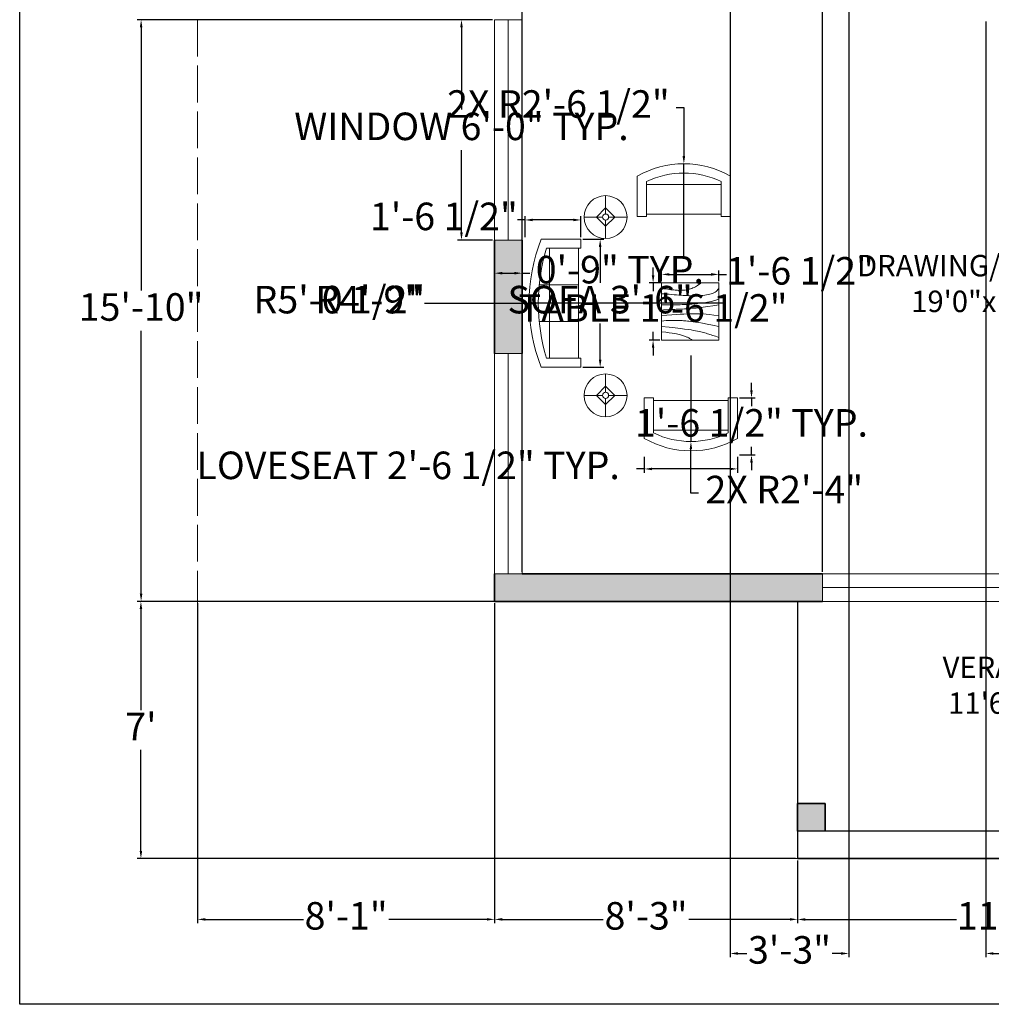
# Model space of a CAD drawing. Units: inches. Extents: x 1942 to 2601, y 2026 to 2623.
# Tile 1 of 5: x 1942 to 2259, y 2026 to 2348. Entities that reach past the tile are written whole.
import ezdxf

# ---------------------------------------------------------------- set-up
doc = ezdxf.new("R2010")
doc.units = ezdxf.units.IN
doc.linetypes.add('ACAD_ISO02W100', pattern=[15, 12, -3])
for name, color, linetype, lineweight in [('A-ANNO-DIMS', 2, 'Continuous', 18), ('A-ANNO-TTLB', 7, 'Continuous', 25), ('A-AREA-IDEN', 7, 'Continuous', 25), ('A-COLS', 7, 'Continuous', 35), ('A-FLOR', 7, 'Continuous', 25), ('A-FLOR-OTLN', 8, 'ACAD_ISO02W100', 13), ('A-FURN', 8, 'Continuous', 18), ('A-GLAZ', 2, 'Continuous', 18), ('A-WALL', 7, 'Continuous', 35), ('A-WALL-PATT', 7, 'Continuous', 13)]:
    doc.layers.add(name, color=color, linetype=linetype, lineweight=lineweight)
doc.styles.get("Standard").update_dxf_attribs({"font": 'arial.ttf'})
doc.dimstyles.new('ISO-25', dxfattribs={"dimtxt": 9, "dimasz": 2.5, "dimexe": 1.25, "dimexo": 0.625, "dimgap": 2, "dimtad": 0, "dimtih": 1, "dimtoh": 1, "dimdec": 1, "dimlunit": 4, "dimtxsty": 'Standard', "dimcen": 2.5, "dimadec": 0, "dimazin": 0, "dimtfac": 0.5, "dimtdec": 1, "dimtmove": 0, "dimatfit": 3, "dimfxl": 1, "dimarcsym": 0})

# ---------------------------------------------------------------- blocks, each defined once
blk = doc.blocks.new('Sofa - Roundback 7 ft.')
for p, q in [((-36.000027, -34), (-36.000027, -11.4696)), ((-12.00002, -32.4421), (-12.00003, -6.5971)), ((11.99997, -32.4421), (11.99998, -6.5971)), ((35.99998, -34), (35.99998, -11.4696)), ((-35.999844, -13.3819), (35.9998, -13.3819)), ((-36.000027, -32.4421), (35.99998, -32.4421))]:
    blk.add_line(p, q)
for points in [[(-36.000027, -34), (-42.000027, -34), (-42.000027, -8)], [(41.99998, -8), (41.99998, -34), (35.99998, -34)]]:
    blk.add_lwpolyline(points)
for centre, radius, start, end in [((0, -114.25), 114.25, 68.43141, 111.5686), ((-0.00001, -127.1968), 121.1968, 72.72033, 107.2797)]:
    blk.add_arc(centre, radius, start, end)
blk = doc.blocks.new('Sofa - Roundback Loveseat 5 ft.')
for p, q in [((0, -32.44198), (0, -5.99998)), ((-24, -33.99998), (-24, -11.46958)), ((24.00004, -33.99998), (24.00004, -11.46958)), ((-23.9998, -13.38178), (23.99986, -13.38178)), ((-24, -32.44198), (24.00004, -32.44198))]:
    blk.add_line(p, q)
for points in [[(-24, -33.99998), (-30, -33.99998), (-30, -7.99998)], [(30.00004, -7.99998), (30.00004, -33.99998), (24.00004, -33.99998)]]:
    blk.add_lwpolyline(points)
for centre, radius, start, end in [((0, -60.24998), 60.24998, 60.13715, 119.8628), ((0, -61.38438), 55.38444, 64.32083, 115.6792)]:
    blk.add_arc(centre, radius, start, end)
blk = doc.blocks.new('Table - Square Woodgrain 42 x 42 in.')
blk.add_line((0, -42), (42, -42))
for points in [[(0, -4), (1.704, -4.2172), (3.2358, -4.4188), (4.615, -4.604), (5.8615, -4.7721), (6.9951, -4.9224), (8.0357, -5.0541), (9.0031, -5.1667), (9.9171, -5.2594), (10.7951, -5.3316), (11.6445, -5.3836), (12.4702, -5.4157), (13.277, -5.4283), (14.0698, -5.4217), (14.8535, -5.3964), (15.6331, -5.3526), (16.4133, -5.2908), (17.1986, -5.2103), (17.9913, -5.1062), (18.793, -4.9727), (19.6056, -4.8038), (20.4307, -4.5937), (21.2701, -4.3365), (22.1256, -4.0262), (22.9989, -3.6571), (23.888, -3.2272), (24.7756, -2.7516), (25.6408, -2.2491), (26.4624, -1.7387), (27.2195, -1.2395), (27.891, -0.7703), (28.456, -0.3501), (28.8934, 0.002)], [(0, -42), (0, 0), (42, 0), (42, -42)], [(0, -8), (1.8203, -8.1001), (3.6741, -8.2149), (5.5411, -8.3408), (7.4011, -8.4741), (9.2339, -8.6112), (11.0193, -8.7484), (12.7371, -8.8821), (14.3671, -9.0086), (15.8954, -9.1246), (17.3337, -9.2278), (18.6997, -9.3159), (20.0116, -9.387), (21.2871, -9.4389), (22.5442, -9.4696), (23.8008, -9.477), (25.0749, -9.459), (26.3791, -9.4137), (27.7049, -9.3403), (29.0383, -9.2382), (30.3655, -9.1068), (31.6728, -8.9455), (32.9461, -8.7535), (34.1717, -8.5304), (35.3358, -8.2756), (36.4268, -7.9863), (37.443, -7.6521), (38.3849, -7.2603), (39.253, -6.7986), (40.048, -6.2542), (40.7705, -5.6147), (41.421, -4.8674), (42, -4)], [(42, -12), (39.1784, -12.8621), (36.4519, -13.5654), (33.8246, -14.1294), (31.3004, -14.5731), (28.8832, -14.9161), (26.577, -15.1775), (24.3858, -15.3768), (22.3136, -15.5332), (20.3622, -15.6632), (18.5254, -15.7718), (16.7947, -15.8612), (15.1618, -15.9338), (13.6183, -15.9916), (12.1558, -16.0369), (10.7659, -16.0718), (9.4403, -16.0987), (8.1703, -16.1191), (6.9461, -16.1325), (5.7577, -16.1377), (4.595, -16.1335), (3.4479, -16.1188), (2.3064, -16.0924), (1.1604, -16.0532), (0, -16)], [(42, -16), (37.6529, -16.7365), (33.8802, -17.329), (30.6179, -17.7961), (27.8015, -18.1561), (25.3668, -18.4275), (23.2497, -18.6288), (21.3859, -18.7785), (19.7111, -18.8949), (18.1693, -18.9939), (16.7375, -19.0795), (15.401, -19.1534), (14.1449, -19.217), (12.9544, -19.2717), (11.8148, -19.3191), (10.7113, -19.3606), (9.6291, -19.3976), (8.5534, -19.4323), (7.47, -19.4689), (6.3643, -19.5122), (5.222, -19.5672), (4.0288, -19.6386), (2.7703, -19.7313), (1.4321, -19.8501), (0, -20)], [(0, -24), (3.9243, -23.6805), (7.4766, -23.4138), (10.6891, -23.1954), (13.5943, -23.0205), (16.2247, -22.8847), (18.6125, -22.7832), (20.7903, -22.7116), (22.7903, -22.6651), (24.6563, -22.642), (26.4764, -22.6507), (28.35, -22.7024), (30.3766, -22.8084), (32.6555, -22.98), (35.2861, -23.2283), (38.3678, -23.5645), (42, -24)], [(42, -32), (37.392, -31.017), (33.4585, -30.2231), (30.1291, -29.5949), (27.3334, -29.109), (25.0009, -28.742), (23.0612, -28.4707), (21.4439, -28.2716), (20.0786, -28.1215), (18.8998, -28.0002), (17.8609, -27.9014), (16.9206, -27.8219), (16.0371, -27.7588), (15.1691, -27.709), (14.2748, -27.6693), (13.3128, -27.6368), (12.2415, -27.6083), (11.0295, -27.5824), (9.6867, -27.5643), (8.233, -27.5608), (6.6884, -27.5787), (5.0728, -27.6248), (3.4062, -27.7058), (1.7086, -27.8286), (0, -28)], [(0, -32), (5.4026, -32.5358), (9.9494, -33.019), (13.7424, -33.4553), (16.8834, -33.8505), (19.4743, -34.2106), (21.6171, -34.5413), (23.4136, -34.8486), (24.9657, -35.1382), (26.3614, -35.4156), (27.6332, -35.6841), (28.7995, -35.9467), (29.8788, -36.2064), (30.8897, -36.4661), (31.8507, -36.7288), (32.7802, -36.9973), (33.6968, -37.2747), (34.6175, -37.5635), (35.5531, -37.8651), (36.5128, -38.1805), (37.506, -38.5108), (38.5421, -38.8568), (39.6302, -39.2197), (40.7797, -39.6004), (42, -40)], [(0, -36), (3.0098, -36.2857), (5.5354, -36.5643), (7.6368, -36.8359), (9.374, -37.1009), (10.807, -37.3597), (11.9957, -37.6126), (13.0002, -37.8599), (13.8804, -38.102), (14.6874, -38.3393), (15.4365, -38.5729), (16.1338, -38.8041), (16.7858, -39.0341), (17.3987, -39.264), (17.9787, -39.4952), (18.5322, -39.7288), (19.0655, -39.9662), (19.5832, -40.2081), (20.0842, -40.4544), (20.5657, -40.7046), (21.0249, -40.9581), (21.459, -41.2144), (21.8653, -41.4731), (22.2409, -41.7335), (22.5831, -41.9951)]]:
    blk.add_lwpolyline(points)
blk = doc.blocks.new('Lamp - Table')
for p, q in [((0, 7), (0, 1)), ((-1, 0), (-7, 0)), ((0, 3), (-3, 0)), ((-3, 0), (0, -3)), ((3, 0), (0, 3)), ((0, -3), (3, 0)), ((1, 0), (7, 0)), ((0, -1), (0, -7))]:
    blk.add_line(p, q)
for radius in [7, 1]:
    blk.add_circle((0, 0), radius)
blk = doc.blocks.new('*D17')
at = {"layer": 'A-ANNO-DIMS', "color": 0, "lineweight": -2, "transparency": 16777216}
for p, q in [((2096.19, 2347.91), (1980.09, 2347.91)), ((1981.34, 2345.41), (1981.34, 2259.51)), ((1981.34, 2160.41), (1981.34, 2246.32)), ((2096.19, 2157.91), (1980.09, 2157.91))]:
    blk.add_line(p, q, dxfattribs=at)
at = {"layer": 'A-ANNO-DIMS', "color": 0, "transparency": 16777216}
for points in [[(1980.92, 2345.41), (1981.75, 2345.41), (1981.34, 2347.91)], [(1980.92, 2160.41), (1981.75, 2160.41), (1981.34, 2157.91)]]:
    blk.add_solid(points, dxfattribs=at)
at = {"layer": 'Defpoints', "color": 0, "transparency": 16777216}
for p in [(2096.82, 2347.91), (1981.34, 2157.91), (2096.82, 2157.91)]:
    blk.add_point(p, dxfattribs=at)
at = {"layer": 'A-ANNO-DIMS', "color": 0, "transparency": 16777216, "insert": (1981.34, 2252.91), "char_height": 9, "attachment_point": 5}
blk.add_mtext('15\'-10"', dxfattribs=at)
blk = doc.blocks.new('*D18')
at = {"layer": 'A-ANNO-DIMS', "color": 0, "lineweight": -2, "transparency": 16777216}
for p, q in [((2195.19, 2157.91), (1980.03, 2157.91)), ((1981.28, 2155.41), (1981.28, 2122.41)), ((1981.28, 2076.41), (1981.28, 2109.41)), ((2195.19, 2073.91), (1980.03, 2073.91))]:
    blk.add_line(p, q, dxfattribs=at)
at = {"layer": 'A-ANNO-DIMS', "color": 0, "transparency": 16777216}
for points in [[(1980.87, 2155.41), (1981.7, 2155.41), (1981.28, 2157.91)], [(1980.87, 2076.41), (1981.7, 2076.41), (1981.28, 2073.91)]]:
    blk.add_solid(points, dxfattribs=at)
at = {"layer": 'Defpoints', "color": 0, "transparency": 16777216}
for p in [(2195.82, 2157.91), (1981.28, 2073.91), (2195.82, 2073.91)]:
    blk.add_point(p, dxfattribs=at)
at = {"layer": 'A-ANNO-DIMS', "color": 0, "transparency": 16777216, "insert": (1981.28, 2115.91), "char_height": 9, "attachment_point": 5}
blk.add_mtext("7'", dxfattribs=at)
blk = doc.blocks.new('*D19')
at = {"layer": 'A-ANNO-DIMS', "color": 0, "lineweight": -2, "transparency": 16777216}
for p, q in [((1999.82, 2157.29), (1999.82, 2052.8)), ((2096.82, 2157.29), (2096.82, 2052.8)), ((2002.32, 2054.05), (2034.35, 2054.05)), ((2094.32, 2054.05), (2062.29, 2054.05))]:
    blk.add_line(p, q, dxfattribs=at)
at = {"layer": 'A-ANNO-DIMS', "color": 0, "transparency": 16777216}
for points in [[(2002.32, 2054.47), (2002.32, 2053.64), (1999.82, 2054.05)], [(2094.32, 2054.47), (2094.32, 2053.64), (2096.82, 2054.05)]]:
    blk.add_solid(points, dxfattribs=at)
at = {"layer": 'Defpoints', "color": 0, "transparency": 16777216}
for p in [(1999.82, 2157.91), (2096.82, 2157.91), (2096.82, 2054.05)]:
    blk.add_point(p, dxfattribs=at)
at = {"layer": 'A-ANNO-DIMS', "color": 0, "transparency": 16777216, "insert": (2048.32, 2054.05), "char_height": 9, "attachment_point": 5}
blk.add_mtext('8\'-1"', dxfattribs=at)
blk = doc.blocks.new('*D20')
at = {"layer": 'A-ANNO-DIMS', "color": 0, "lineweight": -2, "transparency": 16777216}
for p, q in [((2096.82, 2073.29), (2096.82, 2052.8)), ((2195.82, 2073.29), (2195.82, 2052.8)), ((2099.32, 2054.05), (2132.35, 2054.05)), ((2193.32, 2054.05), (2160.29, 2054.05))]:
    blk.add_line(p, q, dxfattribs=at)
at = {"layer": 'A-ANNO-DIMS', "color": 0, "transparency": 16777216}
for points in [[(2099.32, 2054.47), (2099.32, 2053.64), (2096.82, 2054.05)], [(2193.32, 2054.47), (2193.32, 2053.64), (2195.82, 2054.05)]]:
    blk.add_solid(points, dxfattribs=at)
at = {"layer": 'Defpoints', "color": 0, "transparency": 16777216}
for p in [(2096.82, 2073.91), (2195.82, 2073.91), (2195.82, 2054.05)]:
    blk.add_point(p, dxfattribs=at)
at = {"layer": 'A-ANNO-DIMS', "color": 0, "transparency": 16777216, "insert": (2146.32, 2054.05), "char_height": 9, "attachment_point": 5}
blk.add_mtext('8\'-3"', dxfattribs=at)
blk = doc.blocks.new('*D21')
at = {"layer": 'A-ANNO-DIMS', "color": 0, "lineweight": -2, "transparency": 16777216}
for p, q in [((2195.82, 2073.29), (2195.82, 2052.78)), ((2333.82, 2073.29), (2333.82, 2052.78)), ((2198.32, 2054.03), (2247.78, 2054.03)), ((2331.32, 2054.03), (2281.85, 2054.03))]:
    blk.add_line(p, q, dxfattribs=at)
at = {"layer": 'A-ANNO-DIMS', "color": 0, "transparency": 16777216}
for points in [[(2198.32, 2054.45), (2198.32, 2053.61), (2195.82, 2054.03)], [(2331.32, 2054.45), (2331.32, 2053.61), (2333.82, 2054.03)]]:
    blk.add_solid(points, dxfattribs=at)
at = {"layer": 'Defpoints', "color": 0, "transparency": 16777216}
for p in [(2195.82, 2073.91), (2333.82, 2073.91), (2333.82, 2054.03)]:
    blk.add_point(p, dxfattribs=at)
at = {"layer": 'A-ANNO-DIMS', "color": 0, "transparency": 16777216, "insert": (2264.82, 2054.03), "char_height": 9, "attachment_point": 5}
blk.add_mtext('11\'-6"', dxfattribs=at)
blk = doc.blocks.new('WIN-72IN')
for p, q in [((0, 0), (0, 9)), ((0, 9), (72, 9)), ((72, 0), (72, 9)), ((0, 4.5), (72, 4.5)), ((0, 0), (72, 0))]:
    blk.add_line(p, q)
blk = doc.blocks.new('*D31')
at = {"layer": 'A-ANNO-DIMS', "color": 0, "lineweight": -2, "transparency": 16777216}
for p, q in [((2096.19, 2347.91), (2084.77, 2347.91)), ((2086.02, 2345.41), (2086.02, 2318.57)), ((2086.02, 2278.41), (2086.02, 2305.26)), ((2096.19, 2275.91), (2084.77, 2275.91))]:
    blk.add_line(p, q, dxfattribs=at)
at = {"layer": 'A-ANNO-DIMS', "color": 0, "transparency": 16777216}
for points in [[(2085.6, 2345.41), (2086.44, 2345.41), (2086.02, 2347.91)], [(2085.6, 2278.41), (2086.44, 2278.41), (2086.02, 2275.91)]]:
    blk.add_solid(points, dxfattribs=at)
at = {"layer": 'Defpoints', "color": 0, "transparency": 16777216}
for p in [(2096.82, 2347.91), (2086.02, 2275.91), (2096.82, 2275.91)]:
    blk.add_point(p, dxfattribs=at)
at = {"layer": 'A-ANNO-DIMS', "color": 0, "transparency": 16777216, "insert": (2086.02, 2311.91), "char_height": 9, "attachment_point": 5}
blk.add_mtext('WINDOW 6\'-0" TYP.', dxfattribs=at)
blk = doc.blocks.new('*D32')
at = {"layer": 'A-ANNO-DIMS', "color": 0, "lineweight": -2, "transparency": 16777216}
for p, q in [((2096.82, 2275.29), (2096.82, 2263.86)), ((2105.82, 2275.29), (2105.82, 2263.86)), ((2099.32, 2265.11), (2103.32, 2265.11)), ((2105.82, 2265.11), (2108.32, 2265.11))]:
    blk.add_line(p, q, dxfattribs=at)
at = {"layer": 'A-ANNO-DIMS', "color": 0, "transparency": 16777216}
for points in [[(2099.32, 2265.53), (2099.32, 2264.7), (2096.82, 2265.11)], [(2103.32, 2265.53), (2103.32, 2264.7), (2105.82, 2265.11)]]:
    blk.add_solid(points, dxfattribs=at)
at = {"layer": 'Defpoints', "color": 0, "transparency": 16777216}
for p in [(2096.82, 2275.91), (2105.82, 2275.91), (2105.82, 2265.11)]:
    blk.add_point(p, dxfattribs=at)
at = {"layer": 'A-ANNO-DIMS', "color": 0, "transparency": 16777216, "insert": (2137.75, 2265.11), "char_height": 9, "attachment_point": 5}
blk.add_mtext('0\'-9" TYP.', dxfattribs=at)
blk = doc.blocks.new('*D43')
at = {"layer": 'A-ANNO-DIMS', "color": 0, "lineweight": -2, "transparency": 16777216}
for p, q in [((2145.75, 2205.12), (2145.75, 2199.93)), ((2176.2, 2205.12), (2176.2, 2199.93)), ((2145.75, 2201.18), (2143.25, 2201.18)), ((2173.7, 2201.18), (2148.25, 2201.18))]:
    blk.add_line(p, q, dxfattribs=at)
at = {"layer": 'A-ANNO-DIMS', "color": 0, "transparency": 16777216}
for points in [[(2148.25, 2201.6), (2148.25, 2200.77), (2145.75, 2201.18)], [(2173.7, 2201.6), (2173.7, 2200.77), (2176.2, 2201.18)]]:
    blk.add_solid(points, dxfattribs=at)
at = {"layer": 'Defpoints', "color": 0, "transparency": 16777216}
for p in [(2145.75, 2205.75), (2176.2, 2205.75), (2145.75, 2201.18)]:
    blk.add_point(p, dxfattribs=at)
at = {"layer": 'A-ANNO-DIMS', "color": 0, "transparency": 16777216, "insert": (2068.6, 2201.18), "char_height": 9, "attachment_point": 5}
blk.add_mtext('LOVESEAT 2\'-6 1/2" TYP.', dxfattribs=at)
blk = doc.blocks.new('*D44')
at = {"layer": 'A-ANNO-DIMS', "color": 0, "lineweight": -2, "transparency": 16777216}
for p, q in [((2180.77, 2226.85), (2180.77, 2229.35)), ((2176.82, 2224.35), (2182.02, 2224.35)), ((2180.77, 2224.35), (2180.77, 2221.71)), ((2180.77, 2205.75), (2180.77, 2208.4)), ((2176.82, 2205.75), (2182.02, 2205.75)), ((2180.77, 2203.25), (2180.77, 2200.75))]:
    blk.add_line(p, q, dxfattribs=at)
at = {"layer": 'A-ANNO-DIMS', "color": 0, "transparency": 16777216}
for points in [[(2180.35, 2226.85), (2181.18, 2226.85), (2180.77, 2224.35)], [(2180.35, 2203.25), (2181.18, 2203.25), (2180.77, 2205.75)]]:
    blk.add_solid(points, dxfattribs=at)
at = {"layer": 'Defpoints', "color": 0, "transparency": 16777216}
for p in [(2176.2, 2224.35), (2176.2, 2205.75), (2180.77, 2205.75)]:
    blk.add_point(p, dxfattribs=at)
at = {"layer": 'A-ANNO-DIMS', "color": 0, "transparency": 16777216, "insert": (2180.77, 2215.05), "char_height": 9, "attachment_point": 5}
blk.add_mtext('1\'-6 1/2" TYP.', dxfattribs=at)
blk = doc.blocks.new('*D45')
at = {"layer": 'A-ANNO-DIMS', "color": 0, "lineweight": -2, "transparency": 16777216}
for p, q in [((2125.68, 2276.22), (2132.58, 2276.22)), ((2131.33, 2273.72), (2131.33, 2261.97)), ((2131.33, 2236.89), (2131.33, 2248.65)), ((2125.68, 2234.39), (2132.58, 2234.39))]:
    blk.add_line(p, q, dxfattribs=at)
at = {"layer": 'A-ANNO-DIMS', "color": 0, "transparency": 16777216}
for points in [[(2130.91, 2273.72), (2131.74, 2273.72), (2131.33, 2276.22)], [(2130.91, 2236.89), (2131.74, 2236.89), (2131.33, 2234.39)]]:
    blk.add_solid(points, dxfattribs=at)
at = {"layer": 'Defpoints', "color": 0, "transparency": 16777216}
for p in [(2125.05, 2276.22), (2131.33, 2276.22), (2125.05, 2234.39)]:
    blk.add_point(p, dxfattribs=at)
at = {"layer": 'A-ANNO-DIMS', "color": 0, "transparency": 16777216, "insert": (2131.33, 2255.31), "char_height": 9, "attachment_point": 5}
blk.add_mtext('SOFA 3\'-6"', dxfattribs=at)
blk = doc.blocks.new('*D46')
at = {"layer": 'A-ANNO-DIMS', "color": 0, "lineweight": -2, "transparency": 16777216}
for p, q in [((2106.79, 2276.85), (2106.79, 2283.75)), ((2125.05, 2276.85), (2125.05, 2283.75)), ((2106.79, 2282.5), (2104.29, 2282.5)), ((2122.55, 2282.5), (2109.29, 2282.5))]:
    blk.add_line(p, q, dxfattribs=at)
at = {"layer": 'A-ANNO-DIMS', "color": 0, "transparency": 16777216}
for points in [[(2109.29, 2282.92), (2109.29, 2282.08), (2106.79, 2282.5)], [(2122.55, 2282.92), (2122.55, 2282.08), (2125.05, 2282.5)]]:
    blk.add_solid(points, dxfattribs=at)
at = {"layer": 'Defpoints', "color": 0, "transparency": 16777216}
for p in [(2106.79, 2282.5), (2106.79, 2276.22), (2125.05, 2276.22)]:
    blk.add_point(p, dxfattribs=at)
at = {"layer": 'A-ANNO-DIMS', "color": 0, "transparency": 16777216, "insert": (2080.26, 2282.5), "char_height": 9, "attachment_point": 5}
blk.add_mtext('1\'-6 1/2"', dxfattribs=at)
blk = doc.blocks.new('*D47')
at = {"layer": 'A-ANNO-DIMS', "color": 0, "lineweight": -2, "transparency": 16777216}
for p, q in [((2148.62, 2264.42), (2148.62, 2266.92)), ((2150.79, 2261.92), (2147.37, 2261.92)), ((2148.62, 2261.92), (2148.62, 2259.24)), ((2148.62, 2243.26), (2148.62, 2245.93)), ((2150.79, 2243.26), (2147.37, 2243.26)), ((2148.62, 2240.76), (2148.62, 2238.26))]:
    blk.add_line(p, q, dxfattribs=at)
at = {"layer": 'A-ANNO-DIMS', "color": 0, "transparency": 16777216}
for points in [[(2148.2, 2264.42), (2149.04, 2264.42), (2148.62, 2261.92)], [(2148.2, 2240.76), (2149.04, 2240.76), (2148.62, 2243.26)]]:
    blk.add_solid(points, dxfattribs=at)
at = {"layer": 'Defpoints', "color": 0, "transparency": 16777216}
for p in [(2148.62, 2261.92), (2151.42, 2261.92), (2151.42, 2243.26)]:
    blk.add_point(p, dxfattribs=at)
at = {"layer": 'A-ANNO-DIMS', "color": 0, "transparency": 16777216, "insert": (2148.62, 2252.59), "char_height": 9, "attachment_point": 5}
blk.add_mtext('TABLE 1\'-6 1/2"', dxfattribs=at)
blk = doc.blocks.new('*D48')
at = {"layer": 'A-ANNO-DIMS', "color": 0, "lineweight": -2, "transparency": 16777216}
for p, q in [((2151.42, 2262.54), (2151.42, 2265.97)), ((2153.92, 2264.72), (2167.58, 2264.72)), ((2170.08, 2262.54), (2170.08, 2265.97)), ((2170.08, 2264.72), (2172.58, 2264.72))]:
    blk.add_line(p, q, dxfattribs=at)
at = {"layer": 'A-ANNO-DIMS', "color": 0, "transparency": 16777216}
for points in [[(2153.92, 2265.13), (2153.92, 2264.3), (2151.42, 2264.72)], [(2167.58, 2265.13), (2167.58, 2264.3), (2170.08, 2264.72)]]:
    blk.add_solid(points, dxfattribs=at)
at = {"layer": 'Defpoints', "color": 0, "transparency": 16777216}
for p in [(2170.08, 2264.72), (2151.42, 2261.92), (2170.08, 2261.92)]:
    blk.add_point(p, dxfattribs=at)
at = {"layer": 'A-ANNO-DIMS', "color": 0, "transparency": 16777216, "insert": (2196.6, 2264.72), "char_height": 9, "attachment_point": 5}
blk.add_mtext('1\'-6 1/2"', dxfattribs=at)
blk = doc.blocks.new('*D66')
at = {"layer": 'A-ANNO-DIMS', "color": 0, "lineweight": -2, "transparency": 16777216}
for p, q in [((2105.82, 2167.54), (2105.82, 2580.37)), ((2203.92, 2167.54), (2203.92, 2580.37)), ((2108.32, 2579.12), (2140.9, 2579.12)), ((2201.42, 2579.12), (2168.84, 2579.12))]:
    blk.add_line(p, q, dxfattribs=at)
at = {"layer": 'A-ANNO-DIMS', "color": 0, "transparency": 16777216}
for points in [[(2108.32, 2579.54), (2108.32, 2578.7), (2105.82, 2579.12)], [(2201.42, 2579.54), (2201.42, 2578.7), (2203.92, 2579.12)]]:
    blk.add_solid(points, dxfattribs=at)
at = {"layer": 'Defpoints', "color": 0, "transparency": 16777216}
for p in [(2203.92, 2579.12), (2105.82, 2166.91), (2203.92, 2166.91)]:
    blk.add_point(p, dxfattribs=at)
at = {"layer": 'A-ANNO-DIMS', "color": 0, "transparency": 16777216, "insert": (2154.87, 2579.12), "char_height": 9, "attachment_point": 5}
blk.add_mtext('8\'-2"', dxfattribs=at)
blk = doc.blocks.new('*D69')
at = {"layer": 'A-ANNO-DIMS', "color": 0, "lineweight": -2, "transparency": 16777216}
for p, q in [((2257.32, 2347.29), (2257.32, 2041.66)), ((2342.82, 2347.29), (2342.82, 2041.66)), ((2259.82, 2042.91), (2275.66, 2042.91)), ((2340.32, 2042.91), (2324.48, 2042.91))]:
    blk.add_line(p, q, dxfattribs=at)
at = {"layer": 'A-ANNO-DIMS', "color": 0, "transparency": 16777216}
for points in [[(2259.82, 2043.33), (2259.82, 2042.5), (2257.32, 2042.91)], [(2340.32, 2043.33), (2340.32, 2042.5), (2342.82, 2042.91)]]:
    blk.add_solid(points, dxfattribs=at)
at = {"layer": 'Defpoints', "color": 0, "transparency": 16777216}
for p in [(2257.32, 2347.91), (2342.82, 2347.91), (2342.82, 2042.91)]:
    blk.add_point(p, dxfattribs=at)
at = {"layer": 'A-ANNO-DIMS', "color": 0, "transparency": 16777216, "insert": (2300.07, 2042.91), "char_height": 9, "attachment_point": 5}
blk.add_mtext('7\'-1 1/2"', dxfattribs=at)
blk = doc.blocks.new('*D71')
at = {"layer": 'A-ANNO-DIMS', "color": 0, "lineweight": -2, "transparency": 16777216}
for p, q in [((2173.82, 2398.29), (2173.82, 2041.66)), ((2212.57, 2398.29), (2212.57, 2041.66)), ((2176.32, 2042.91), (2179.24, 2042.91)), ((2210.07, 2042.91), (2207.15, 2042.91))]:
    blk.add_line(p, q, dxfattribs=at)
at = {"layer": 'A-ANNO-DIMS', "color": 0, "transparency": 16777216}
for points in [[(2176.32, 2043.33), (2176.32, 2042.5), (2173.82, 2042.91)], [(2210.07, 2043.33), (2210.07, 2042.5), (2212.57, 2042.91)]]:
    blk.add_solid(points, dxfattribs=at)
at = {"layer": 'Defpoints', "color": 0, "transparency": 16777216}
for p in [(2173.82, 2398.91), (2212.57, 2398.91), (2212.57, 2042.91)]:
    blk.add_point(p, dxfattribs=at)
at = {"layer": 'A-ANNO-DIMS', "color": 0, "transparency": 16777216, "insert": (2193.19, 2042.91), "char_height": 9, "attachment_point": 5}
blk.add_mtext('3\'-3"', dxfattribs=at)
blk = doc.blocks.new('*D81')
at = {"layer": 'A-ANNO-DIMS', "color": 0, "lineweight": -2, "transparency": 16777216}
for p, q in [((2074.89, 2255.31), (2108.6, 2255.31)), ((2171.47, 2255.31), (2111.1, 2255.31))]:
    blk.add_line(p, q, dxfattribs=at)
at = {"layer": 'A-ANNO-DIMS', "color": 0, "transparency": 16777216}
blk.add_solid([(2108.6, 2255.72), (2108.6, 2254.89), (2111.1, 2255.31)], dxfattribs=at)
at = {"layer": 'Defpoints', "color": 0, "transparency": 16777216}
for p in [(2111.1, 2255.31), (2171.47, 2255.31)]:
    blk.add_point(p, dxfattribs=at)
at = {"layer": 'A-ANNO-DIMS', "color": 0, "transparency": 16777216, "insert": (2046.13, 2255.31), "char_height": 9, "attachment_point": 5}
blk.add_mtext('R5\'-0 1/2"', dxfattribs=at)
blk = doc.blocks.new('*D82')
at = {"layer": 'A-ANNO-DIMS', "color": 0, "lineweight": -2, "transparency": 16777216}
for p, q in [((2073.97, 2255.31), (2105.62, 2255.31)), ((2165.02, 2255.31), (2108.12, 2255.31))]:
    blk.add_line(p, q, dxfattribs=at)
at = {"layer": 'A-ANNO-DIMS', "color": 0, "transparency": 16777216}
blk.add_solid([(2105.62, 2255.72), (2105.62, 2254.89), (2108.12, 2255.31)], dxfattribs=at)
at = {"layer": 'Defpoints', "color": 0, "transparency": 16777216}
for p in [(2108.12, 2255.31), (2165.02, 2255.31)]:
    blk.add_point(p, dxfattribs=at)
at = {"layer": 'A-ANNO-DIMS', "color": 0, "transparency": 16777216, "insert": (2055.7, 2255.31), "char_height": 9, "attachment_point": 5}
blk.add_mtext('R4\'-9"', dxfattribs=at)
blk = doc.blocks.new('*D83')
at = {"layer": 'A-ANNO-DIMS', "color": 0, "lineweight": -2, "transparency": 16777216}
for p, q in [((2156.18, 2319.2), (2158.68, 2319.2)), ((2158.68, 2319.2), (2158.68, 2303.36)), ((2158.68, 2270.28), (2158.68, 2300.86))]:
    blk.add_line(p, q, dxfattribs=at)
at = {"layer": 'A-ANNO-DIMS', "color": 0, "transparency": 16777216}
blk.add_solid([(2159.09, 2303.36), (2158.26, 2303.36), (2158.68, 2300.86)], dxfattribs=at)
at = {"layer": 'Defpoints', "color": 0, "transparency": 16777216}
for p in [(2158.68, 2300.86), (2158.68, 2270.28)]:
    blk.add_point(p, dxfattribs=at)
at = {"layer": 'A-ANNO-DIMS', "color": 0, "transparency": 16777216, "insert": (2117.68, 2319.2), "char_height": 9, "attachment_point": 5}
blk.add_mtext('2X R2\'-6 1/2"', dxfattribs=at)
blk = doc.blocks.new('*D84')
at = {"layer": 'A-ANNO-DIMS', "color": 0, "lineweight": -2, "transparency": 16777216}
for p, q in [((2160.98, 2238.25), (2160.98, 2210.15)), ((2160.98, 2193.28), (2160.98, 2207.65)), ((2163.48, 2193.28), (2160.98, 2193.28))]:
    blk.add_line(p, q, dxfattribs=at)
at = {"layer": 'A-ANNO-DIMS', "color": 0, "transparency": 16777216}
blk.add_solid([(2161.39, 2207.65), (2160.56, 2207.65), (2160.98, 2210.15)], dxfattribs=at)
at = {"layer": 'Defpoints', "color": 0, "transparency": 16777216}
for p in [(2160.98, 2238.25), (2160.98, 2210.15)]:
    blk.add_point(p, dxfattribs=at)
at = {"layer": 'A-ANNO-DIMS', "color": 0, "transparency": 16777216, "insert": (2191.49, 2193.28), "char_height": 9, "attachment_point": 5}
blk.add_mtext('2X R2\'-4"', dxfattribs=at)

msp = doc.modelspace()

# ---------------------------------------------------------------- hatches: boundary and pattern name
at = {"layer": 'A-WALL-PATT'}
h = msp.add_hatch(color=256, dxfattribs=at)
h.dxf.hatch_style = 1
h.paths.add_polyline_path([(2483.82, 2264.91), (2474.82, 2264.91), (2474.82, 2259.91), (2426.82, 2259.91), (2426.82, 2261.08), (2420.82, 2261.08), (2420.82, 2259.91), (2380.37, 2259.91, -0.055385), (2380.37, 2250.91), (2474.82, 2250.91), (2474.82, 2202.91), (2483.82, 2202.91)])
h.paths.add_polyline_path([(2483.82, 2130.91), (2474.82, 2130.91), (2474.82, 2082.91), (2444.82, 2082.91), (2444.82, 2073.91), (2483.82, 2073.91)])
h.paths.add_polyline_path([(2372.82, 2082.91), (2342.82, 2082.91), (2342.82, 2250.91), (2344.37, 2250.91), (2344.37, 2259.91), (2342.82, 2259.91), (2342.82, 2293.91), (2333.82, 2293.91), (2333.82, 2259.91), (2333.82, 2250.91), (2333.82, 2166.91), (2332.02, 2166.91), (2332.02, 2157.91), (2333.82, 2157.91), (2333.82, 2082.91), (2333.82, 2073.91), (2372.82, 2073.91)])
h.paths.add_polyline_path([(2204.82, 2091.91), (2195.82, 2091.91), (2195.82, 2082.91), (2204.82, 2082.91)])
h.paths.add_polyline_path([(2284.02, 2166.91), (2275.92, 2166.91), (2275.92, 2157.91), (2284.02, 2157.91)])
h.paths.add_polyline_path([(2203.92, 2166.91), (2195.82, 2166.91), (2105.82, 2166.91), (2096.82, 2166.91), (2096.82, 2157.91), (2105.82, 2157.91), (2195.82, 2157.91), (2203.92, 2157.91)])
h.paths.add_polyline_path([(2105.82, 2275.91), (2096.82, 2275.91), (2096.82, 2250.91), (2096.82, 2238.91), (2105.82, 2238.91), (2105.82, 2250.91)])

# ---------------------------------------------------------------- linework, layer by layer
at = {"layer": 'A-ANNO-TTLB'}
msp.add_lwpolyline([(1941.67, 2623.37), (2601.3, 2623.37), (2601.3, 2026.31), (1941.67, 2026.31)], close=True, dxfattribs=at)
at = {"layer": 'A-COLS'}
for p, q in [((2195.82, 2082.91), (2195.82, 2091.91)), ((2195.82, 2091.91), (2204.82, 2091.91)), ((2204.82, 2091.91), (2204.82, 2082.91))]:
    msp.add_line(p, q, dxfattribs=at)
at = {"layer": 'A-FLOR'}
for p, q in [((2195.82, 2157.91), (2195.82, 2082.91)), ((2333.82, 2082.91), (2195.82, 2082.91)), ((2195.82, 2082.91), (2195.82, 2073.91))]:
    msp.add_line(p, q, dxfattribs=at)
at = {"layer": 'A-FLOR-OTLN'}
for p in [(1999.82, 2347.91), (2195.82, 2073.91)]:
    msp.add_line(p, (1999.82, 2073.91), dxfattribs=at)
at = {"layer": 'A-WALL'}
for p, q in [((2096.82, 2250.91), (2096.82, 2275.91)), ((2105.82, 2250.91), (2105.82, 2275.91)), ((2096.82, 2250.91), (2096.82, 2238.91)), ((2105.82, 2250.91), (2105.82, 2238.91)), ((2096.82, 2166.91), (2096.82, 2157.91)), ((2195.82, 2166.91), (2105.82, 2166.91)), ((2203.92, 2166.91), (2195.82, 2166.91)), ((2105.82, 2157.91), (2096.82, 2157.91)), ((2195.82, 2157.91), (2105.82, 2157.91)), ((2203.92, 2157.91), (2195.82, 2157.91)), ((2372.82, 2073.91), (2195.82, 2073.91))]:
    msp.add_line(p, q, dxfattribs=at)

# ---------------------------------------------------------------- block references
at = {"layer": 'A-FURN'}
for name, p, xscale, yscale, zscale in [('Sofa - Roundback Loveseat 5 ft.', (2158.68, 2300.86), 0.5074318559263169, 0.5074318559263169, 0.5074318559263169), ('Table - Square Woodgrain 42 x 42 in.', (2151.42, 2261.92), 0.4442528932482269, 0.4442528932482269, 0.4442528932482269)]:
    msp.add_blockref(name, p, dxfattribs=dict(at, xscale=xscale, yscale=yscale, zscale=zscale))
for p in [(2133.1, 2283.44), (2133.1, 2225.21)]:
    msp.add_blockref('Lamp - Table', p, dxfattribs=at)
for name, p, xscale, yscale, zscale, rotation in [('Sofa - Roundback 7 ft.', (2108.12, 2255.31), 0.4980706007964554, 0.4980706007964554, 0.4980706007964554, 90), ('Sofa - Roundback Loveseat 5 ft.', (2160.98, 2207.1), 0.5074318559263169, 0.5074318559263169, 0.5074318559263169, 180)]:
    msp.add_blockref(name, p, dxfattribs=dict(at, xscale=xscale, yscale=yscale, zscale=zscale, rotation=rotation))
at = {"layer": 'A-GLAZ'}
for p, rotation in [((2096.82, 2347.91), 269.9999999999981), ((2105.82, 2166.91), 89.99999999999947), ((2275.92, 2166.91), 180)]:
    msp.add_blockref('WIN-72IN', p, dxfattribs=dict(at, rotation=rotation))

# ---------------------------------------------------------------- texts
at = {"layer": 'A-AREA-IDEN', "char_height": 7, "attachment_point": 1}
for s, width, insert in [('\\pxqc;{\\fArial|b1|i0|c0|p34;DRAWING/DINNING\\P19\'0"x14\'0"}', 128.6303, (2194.11, 2271.08)), ('\\pxqc;{\\fArial|b1|i0|c0|p34;VERANDAH\\P11\'6"x7\'0"}', 112.3172, (2211.67, 2139.87))]:
    msp.add_mtext_dynamic_manual_height_columns(s, width=width, gutter_width=12.5, heights=[0], dxfattribs=dict(at, insert=insert))

# ---------------------------------------------------------------- dimensions: what is measured, and where the dimension line sits
at = {"layer": 'A-ANNO-DIMS'}
for base, p1, p2, override, picture, middle in [((2203.92, 2579.12), (2105.82, 2166.91), (2203.92, 2166.91), {"dimdec": 1, "dimlfac": 1, "dimrnd": 0, "dimzin": 1, "dimdsep": 46, "dimlunit": 4, "dimfrac": 2}, '*D66', (2154.87, 2579.12)), ((2212.569724, 2042.91449), (2173.819724, 2398.91449), (2212.569724, 2398.91449), {"dimdec": 1, "dimlfac": 1, "dimrnd": 0, "dimzin": 1, "dimdsep": 46, "dimlunit": 4, "dimfrac": 2}, '*D71', (2193.194724, 2042.91449)), ((2342.82, 2042.91), (2257.32, 2347.91), (2342.82, 2347.91), {"dimdec": 1, "dimlfac": 1, "dimrnd": 0, "dimzin": 1, "dimdsep": 46, "dimlunit": 4, "dimfrac": 2}, '*D69', (2300.07, 2042.91)), ((2170.08, 2264.72), (2151.42, 2261.92), (2170.08, 2261.92), {"dimdec": 1, "dimlfac": 1, "dimrnd": 0, "dimzin": 1, "dimdsep": 46, "dimlunit": 4, "dimfrac": 2}, '*D48', (2196.6, 2264.72)), ((2096.82, 2054.05), (1999.82, 2157.91), (2096.82, 2157.91), {"dimclrd": 0, "dimclre": 0, "dimclrt": 0}, '*D19', (2048.32, 2054.05)), ((2195.82, 2054.05), (2096.82, 2073.91), (2195.82, 2073.91), {"dimclrd": 0, "dimclre": 0, "dimclrt": 0}, '*D20', (2146.32, 2054.05)), ((2333.82, 2054.03), (2195.82, 2073.91), (2333.82, 2073.91), {"dimclrd": 0, "dimclre": 0, "dimclrt": 0}, '*D21', (2264.82, 2054.03))]:
    dim = msp.add_linear_dim(base=base, p1=p1, p2=p2, dimstyle='ISO-25', override=override, dxfattribs=at)
    dim.commit()
    dim.dimension.update_dxf_attribs({"geometry": picture, "text_midpoint": middle})
for base, p1, p2, angle, override, picture, middle in [((1981.34, 2157.91), (2096.82, 2347.91), (2096.82, 2157.91), 90, {"dimclrd": 0, "dimclre": 0, "dimclrt": 0}, '*D17', (1981.34, 2252.91)), ((2106.79, 2282.5), (2125.05, 2276.22), (2106.79, 2276.22), 180, {"dimdec": 1, "dimlfac": 1, "dimrnd": 0, "dimzin": 1, "dimdsep": 46, "dimlunit": 4, "dimfrac": 2}, '*D46', (2080.26, 2282.5)), ((1981.28, 2073.91), (2195.82, 2157.91), (2195.82, 2073.91), 90, {"dimclrd": 0, "dimclre": 0, "dimclrt": 0}, '*D18', (1981.28, 2115.91))]:
    dim = msp.add_linear_dim(base=base, p1=p1, p2=p2, angle=angle, dimstyle='ISO-25', override=override, dxfattribs=at)
    dim.commit()
    dim.dimension.update_dxf_attribs({"geometry": picture, "text_midpoint": middle})
for base, p1, p2, angle, text, picture, middle in [((2086.02, 2275.91), (2096.82, 2347.91), (2096.82, 2275.91), 270, 'WINDOW <> TYP.', '*D31', (2086.02, 2311.91)), ((2131.33, 2276.22), (2125.05, 2234.39), (2125.05, 2276.22), 90, 'SOFA <>', '*D45', (2131.33, 2255.31)), ((2148.62, 2261.92), (2151.42, 2243.26), (2151.42, 2261.92), 90, 'TABLE <>', '*D47', (2148.62, 2252.59)), ((2180.77, 2205.75), (2176.2, 2224.35), (2176.2, 2205.75), 270, '<> TYP.', '*D44', (2180.77, 2215.05)), ((2145.7536, 2201.1818), (2176.1995, 2205.7486), (2145.7536, 2205.7486), 180, 'LOVESEAT <> TYP.', '*D43', (2068.5998, 2201.1818))]:
    dim = msp.add_linear_dim(base=base, p1=p1, p2=p2, angle=angle, text=text, dimstyle='ISO-25', override={"dimdec": 1, "dimlfac": 1, "dimrnd": 0, "dimzin": 1, "dimdsep": 46, "dimlunit": 4, "dimfrac": 2}, dxfattribs=at)
    dim.commit()
    dim.dimension.update_dxf_attribs({"geometry": picture, "text_midpoint": middle})
for center, mpoint, picture, middle in [((2158.68, 2270.28), (2158.68, 2300.86), '*D83', (2117.68, 2319.2)), ((2160.98, 2238.25), (2160.98, 2210.15), '*D84', (2191.49, 2193.28))]:
    dim = msp.add_radius_dim(center=center, mpoint=mpoint, text='2X <>', dimstyle='ISO-25', override={"dimdec": 1, "dimlfac": 1, "dimrnd": 0, "dimzin": 1, "dimdsep": 46, "dimlunit": 4, "dimfrac": 2}, dxfattribs=at)
    dim.commit()
    dim.dimension.update_dxf_attribs({"geometry": picture, "text_midpoint": middle, "dimtype": 164})
dim = msp.add_linear_dim(base=(2105.82, 2265.11), p1=(2096.82, 2275.91), p2=(2105.82, 2275.91), text='<> TYP.', dimstyle='ISO-25', override={"dimdec": 1, "dimlfac": 1, "dimrnd": 0, "dimzin": 1, "dimdsep": 46, "dimlunit": 4, "dimfrac": 2}, dxfattribs=at)
dim.commit()
dim.dimension.update_dxf_attribs({"geometry": '*D32', "text_midpoint": (2137.75, 2265.11)})
for center, mpoint, picture, middle in [((2171.47, 2255.31), (2111.1, 2255.31), '*D81', (2074.89, 2255.31)), ((2165.02, 2255.31), (2108.12, 2255.31), '*D82', (2073.97, 2255.31))]:
    dim = msp.add_radius_dim(center=center, mpoint=mpoint, dimstyle='ISO-25', override={"dimdec": 1, "dimlfac": 1, "dimrnd": 0, "dimzin": 1, "dimdsep": 46, "dimlunit": 4, "dimfrac": 2}, dxfattribs=at)
    dim.commit()
    dim.dimension.update_dxf_attribs({"geometry": picture, "text_midpoint": middle, "dimtype": 164})

doc.saveas('drawing.dxf')
